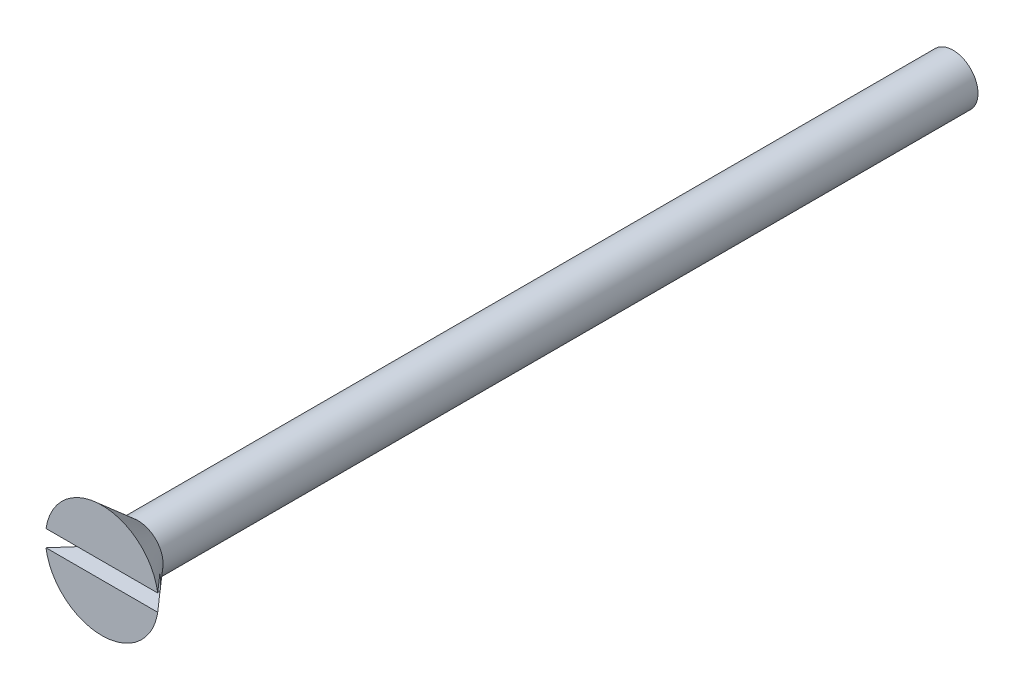
SolidWorks part; units mm, degrees
material "Plain Carbon Steel"
ref_plane "Front Plane" through (0, 0, 0) normal (0, 0, 1) x (1, 0, 0)
ref_plane "Top Plane" through (0, 0, 0) normal (0, 1, 0) x (1, 0, 0)
ref_plane "Right Plane" through (0, 0, 0) normal (1, 0, 0) x (0, 0, -1)
sketch "Shank Profile Ø0.138" plane through (0, 0, 0) normal (0, 0, 1) x (1, 0, 0)
  circle A0 centre (0, 0) radius 1.7526
  dimension "D1" = 3.5052
extrude "Shank Ø0.138 x 2.25" add sketch "Shank Profile Ø0.138" along normal blind 57.15 contours A0
sketch "Countersunk Head Profile" plane through (0, 0, 0) normal (1, 0, 0) x (0, 0, -1)
  line L0 (-57.15, 0) -> (-61.8858, 0) construction
  line L1 (-57.15, 1.7526) -> (-57.15, -1.7526) construction
  line L2 (-57.15, 1.7526) -> (-59.69, 3.9606)
  line L3 (-59.69, 3.9606) -> (-59.69, 0)
  line L4 (-59.69, 0) -> (-57.15, 0)
  line L5 (-57.15, 0) -> (-57.15, 1.7526)
  line L7 (-57.15, 1.7526) -> (-57.15, 8.2159) construction
  dimension "D1" = 41
  dimension "D2" = 2.54
revolve "Countersunk Head 82°" add sketch "Countersunk Head Profile" angle 360 about L4
sketch "Screwdriver Slot Profile" plane through (0, 0, 0) normal (1, 0, 0) x (0, 0, -1)
  line L0 (-59.69, 3.9606) -> (-59.69, -3.9606) construction
  line L1 (-60.96, -0.5843) -> (-58.42, -0.5843)
  line L2 (-60.96, -0.5843) -> (-60.96, 0.5843)
  line L3 (-60.96, 0.5843) -> (-58.42, 0.5843)
  line L4 (-58.42, -0.5843) -> (-58.42, 0.5843)
  line L5 (-60.96, -0.5843) -> (-58.42, 0.5843) construction
  line L6 (-60.96, 0.5843) -> (-58.42, -0.5843) construction
  point P0 (-59.69, 0)
  dimension "D1" = 1.1686
  dimension "0.8" = 2.54
extrude "Screwdriver Slot" cut sketch "Screwdriver Slot Profile" against normal through all both and the other way through all
